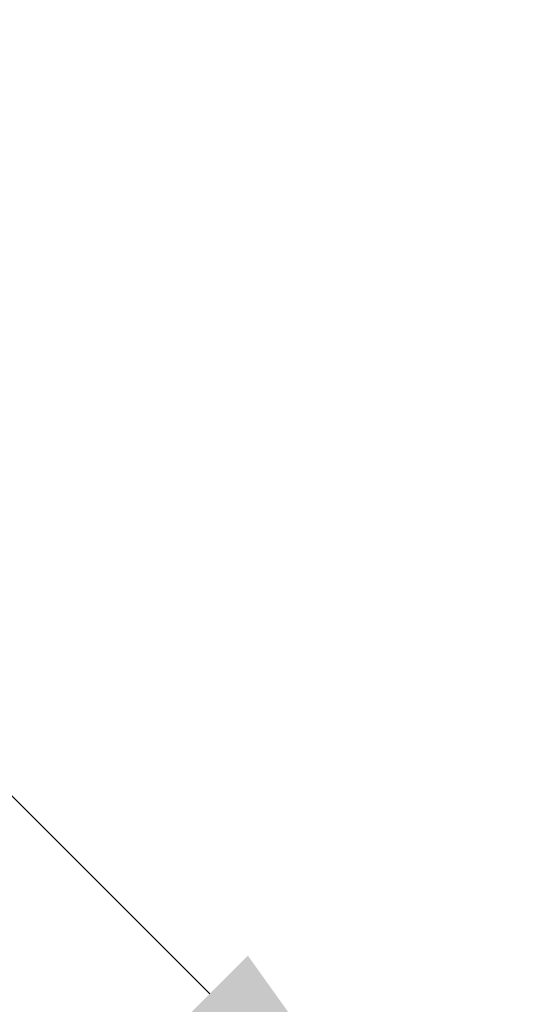
# Model space of a CAD drawing. Units: millimetres. Extents: x 0 to 2267, y 0 to 1823.
# Tile 16 of 256: x 1518.68 to 1525.06, y 1127.19 to 1139.34. Entities that reach past the tile are written whole.
import ezdxf

# ---------------------------------------------------------------- set-up
doc = ezdxf.new("R2010")
doc.units = ezdxf.units.MM
doc.header["$MEASUREMENT"] = 0
for name, color, linetype, lineweight in [('M-DIMS', 2, 'Continuous', 25), ('M-HATC', 252, 'Continuous', 18), ('M-OUTL', 7, 'Continuous', 50)]:
    doc.layers.add(name, color=color, linetype=linetype, lineweight=lineweight)
doc.styles.get("Standard").update_dxf_attribs({"font": 'arial.ttf'})
doc.dimstyles.get("Standard").update_dxf_attribs({"dimtxt": 7, "dimasz": 4, "dimexe": 0.18, "dimexo": 0.0625, "dimgap": 0.09, "dimtad": 0, "dimdec": 0, "dimzin": 0, "dimdsep": 46, "dimtxsty": 'Standard', "dimcen": 0.09, "dimadec": 0, "dimazin": 0, "dimtfac": 1, "dimtdec": 0, "dimtofl": 0, "dimtmove": 0, "dimatfit": 3, "dimfxl": 1, "dimtolj": 1, "dimtzin": 0, "dimarcsym": 0})

# ---------------------------------------------------------------- blocks, each defined once
blk = doc.blocks.new('*D28')
at = {"layer": 'Defpoints', "color": 0, "transparency": 16777216}
for p in [(1523.858, 1124.488), (1530.929, 1117.417)]:
    blk.add_point(p, dxfattribs=at)
at = {"layer": 'M-DIMS', "color": 0, "lineweight": -2, "transparency": 16777216}
for p, q in [((1518.201, 1130.145), (1521.029, 1127.317)), ((1530.929, 1117.327), (1530.929, 1117.507)), ((1530.839, 1117.417), (1531.019, 1117.417))]:
    blk.add_line(p, q, dxfattribs=at)
at = {"layer": 'M-DIMS', "color": 0, "transparency": 16777216}
blk.add_solid([(1521.501, 1127.788), (1520.558, 1126.845), (1523.858, 1124.488)], dxfattribs=at)
at = {"layer": 'M-DIMS', "color": 0, "transparency": 16777216, "insert": (1504.949, 1143.397), "char_height": 7, "attachment_point": 5, "rotation": 314.9998}
blk.add_mtext('\\A1;27X R10', dxfattribs=at)

msp = doc.modelspace()

# ---------------------------------------------------------------- hatches: boundary and pattern name
at = {"layer": 'M-HATC'}
h = msp.add_hatch(color=256, dxfattribs=at)
h.dxf.hatch_style = 1
h.paths.add_polyline_path([(2055.771, 1603.062), (1381.087, 1603.062), (1381.087, 1598.062), (2055.771, 1598.062)])
h.paths.add_polyline_path([(2055.771, 1598.062), (1381.087, 1598.062), (1381.087, 1593.062), (2055.771, 1593.062)])
h.paths.add_polyline_path([(2051.307, 1536.761), (1385.55, 1536.761), (1385.55, 1526.761), (1387.55, 1526.761), (1388.537, 1525.053), (1385.332, 1521.233), (1385.332, 1521.223), (2050.254, 1522.749), (2048.321, 1525.053), (2049.307, 1526.761), (2051.307, 1526.761)])
edge = h.paths.add_edge_path()
edge.add_arc((1847.535, 1379.149), 135, 222.60306, 222.89085, ccw=False)
edge.add_line((1748.166, 1287.766), (1683.092, 1287.766))
edge.add_arc((1583.724, 1379.149), 135, 317.10915, 317.39694, ccw=False)
edge.add_arc((1678.969, 1290.671), 5, 222.8909, 317.1091, ccw=False)
edge.add_arc((1774.213, 1379.149), 135, 222.60306, 222.89085, ccw=False)
edge.add_line((1674.845, 1287.766), (1609.771, 1287.766))
edge.add_arc((1510.403, 1379.149), 135, 317.10915, 317.39694, ccw=False)
edge.add_arc((1605.647, 1290.671), 5, 222.8909, 317.1091, ccw=False)
edge.add_arc((1700.892, 1379.149), 135, 222.60306, 222.89085, ccw=False)
edge.add_line((1601.524, 1287.766), (1536.45, 1287.766))
edge.add_arc((1437.081, 1379.149), 135, 317.10915, 317.39694, ccw=False)
edge.add_arc((1532.326, 1290.671), 5, 222.8909, 317.1091, ccw=False)
edge.add_arc((1627.571, 1379.149), 135, 222.60306, 222.89085, ccw=False)
edge.add_line((1528.203, 1287.766), (1505.929, 1287.766))
edge.add_spline(control_points=[(1505.929, 1287.766), (1504.262, 1287.766), (1504.262, 1282.766), (1505.929, 1282.766)], knot_values=[0, 0, 0, 0, 5, 5, 5, 5], degree=3, periodic=0)
edge.add_line((1505.929, 1282.766), (1930.929, 1282.766))
edge.add_spline(control_points=[(1930.929, 1282.766), (1932.596, 1282.766), (1932.596, 1287.766), (1930.929, 1287.766)], knot_values=[0, 0, 0, 0, 5, 5, 5, 5], degree=3, periodic=0)
edge.add_line((1930.929, 1287.766), (1903.056, 1287.766))
edge.add_arc((1803.688, 1379.149), 135, 317.10915, 317.39694, ccw=False)
edge.add_arc((1898.932, 1290.671), 5, 222.8909, 317.1091, ccw=False)
edge.add_arc((1994.177, 1379.149), 135, 222.60306, 222.89085, ccw=False)
edge.add_line((1894.809, 1287.766), (1829.735, 1287.766))
edge.add_arc((1730.366, 1379.149), 135, 317.10915, 317.39694, ccw=False)
edge.add_arc((1825.611, 1290.671), 5, 222.8909, 317.1091, ccw=False)
edge.add_arc((1920.856, 1379.149), 135, 222.60306, 222.89085, ccw=False)
edge.add_line((1821.487, 1287.766), (1756.413, 1287.766))
edge.add_arc((1657.045, 1379.149), 135, 317.10915, 317.39694, ccw=False)
edge.add_arc((1752.29, 1290.671), 5, 222.8909, 317.1091, ccw=False)
edge = h.paths.add_edge_path()
edge.add_spline(control_points=[(1843.429, 1227.247), (1845.096, 1227.247), (1845.096, 1232.247), (1843.429, 1232.247)], knot_values=[0, 0, 0, 0, 5, 5, 5, 5], degree=3, periodic=0)
edge.add_line((1843.429, 1232.247), (1593.429, 1232.247))
edge.add_spline(control_points=[(1593.429, 1232.247), (1591.762, 1232.247), (1591.762, 1227.247), (1593.429, 1227.247)], knot_values=[0, 0, 0, 0, 5, 5, 5, 5], degree=3, periodic=0)
edge.add_line((1593.429, 1227.247), (1843.429, 1227.247))
h.paths.add_polyline_path([(1905.929, 1127.417), (1530.929, 1127.417, 0.414214), (1520.929, 1117.417), (1530.929, 1117.417), (1915.929, 1117.417, 0.414214)])
edge = h.paths.add_edge_path()
edge.add_arc((1397.086, 1498.408), 12.73, 90.7821, 190.8787, ccw=False)
edge.add_line((1396.912, 1511.136), (1428.01, 1511.349))
edge.add_line((1428.01, 1511.349), (1433.01, 1511.349))
edge.add_line((1433.01, 1511.349), (1434.439, 1511.349))
edge.add_arc((1419.474, 1498.08), 20, 41.561, 74.0821)
edge.add_line((1424.959, 1517.314), (1399.935, 1517.256))
edge.add_spline(control_points=[(1399.931, 1517.256), (1399.884, 1517.213), (1399.833, 1517.169), (1399.777, 1517.124)], knot_values=[11.567499, 11.567499, 11.567499, 11.567499, 11.814249, 11.814249, 11.814249, 11.814249], degree=3, periodic=0)
edge.add_spline(control_points=[(1399.633, 1517.01), (1399.583, 1516.972), (1399.531, 1516.934), (1399.476, 1516.895)], knot_values=[11.167718, 11.167718, 11.167718, 11.167718, 11.365188, 11.365188, 11.365188, 11.365188], degree=3, periodic=0)
edge.add_spline(control_points=[(1399.34, 1516.8), (1399.151, 1516.672), (1398.938, 1516.538), (1398.704, 1516.399)], knot_values=[10.376405, 10.376405, 10.376405, 10.376405, 11.00994, 11.00994, 11.00994, 11.00994], degree=3, periodic=0)
edge.add_spline(control_points=[(1398.657, 1516.372), (1398.579, 1516.326), (1398.498, 1516.28), (1398.415, 1516.233)], knot_values=[10.125175, 10.125175, 10.125175, 10.125175, 10.334406, 10.334406, 10.334406, 10.334406], degree=3, periodic=0)
edge.add_spline(control_points=[(1398.264, 1516.149), (1398.196, 1516.111), (1398.126, 1516.073), (1398.055, 1516.035)], knot_values=[9.832246, 9.832246, 9.832246, 9.832246, 9.999658, 9.999658, 9.999658, 9.999658], degree=3, periodic=0)
edge.add_spline(control_points=[(1397.999, 1516.005), (1397.731, 1515.862), (1397.446, 1515.717), (1397.147, 1515.571)], knot_values=[9.161808, 9.161808, 9.161808, 9.161808, 9.787769, 9.787769, 9.787769, 9.787769], degree=3, periodic=0)
edge.add_spline(control_points=[(1397.147, 1515.571), (1396.842, 1515.423), (1396.522, 1515.274), (1396.191, 1515.126)], knot_values=[8.524455, 8.524455, 8.524455, 8.524455, 9.161808, 9.161808, 9.161808, 9.161808], degree=3, periodic=0)
edge.add_spline(control_points=[(1396.078, 1515.076), (1395.985, 1515.035), (1395.892, 1514.994), (1395.798, 1514.953)], knot_values=[8.275193, 8.275193, 8.275193, 8.275193, 8.451726, 8.451726, 8.451726, 8.451726], degree=3, periodic=0)
edge.add_spline(control_points=[(1395.602, 1514.869), (1395.5, 1514.826), (1395.397, 1514.782), (1395.293, 1514.739)], knot_values=[7.962917, 7.962917, 7.962917, 7.962917, 8.152764, 8.152764, 8.152764, 8.152764], degree=3, periodic=0)
edge.add_spline(control_points=[(1395.212, 1514.706), (1394.828, 1514.547), (1394.435, 1514.393), (1394.036, 1514.244)], knot_values=[7.21254, 7.21254, 7.21254, 7.21254, 7.913148, 7.913148, 7.913148, 7.913148], degree=3, periodic=0)
edge.add_spline(control_points=[(1394.036, 1514.244), (1393.708, 1514.121), (1393.375, 1514.003), (1393.043, 1513.889)], knot_values=[6.633733, 6.633733, 6.633733, 6.633733, 7.21254, 7.21254, 7.21254, 7.21254], degree=3, periodic=0)
edge.add_spline(control_points=[(1392.821, 1513.815), (1392.72, 1513.781), (1392.618, 1513.748), (1392.517, 1513.715)], knot_values=[6.328796, 6.328796, 6.328796, 6.328796, 6.505493, 6.505493, 6.505493, 6.505493], degree=3, periodic=0)
edge.add_spline(control_points=[(1392.517, 1513.715), (1392.319, 1513.652), (1392.121, 1513.59), (1391.924, 1513.531)], knot_values=[5.984605, 5.984605, 5.984605, 5.984605, 6.328796, 6.328796, 6.328796, 6.328796], degree=3, periodic=0)
edge.add_spline(control_points=[(1391.792, 1513.491), (1391.312, 1513.35), (1390.838, 1513.224), (1390.378, 1513.117)], knot_values=[5.066697, 5.066697, 5.066697, 5.066697, 5.907055, 5.907055, 5.907055, 5.907055], degree=3, periodic=0)
edge.add_spline(control_points=[(1390.378, 1513.117), (1390.18, 1513.071), (1389.984, 1513.028), (1389.791, 1512.99)], knot_values=[4.70367, 4.70367, 4.70367, 4.70367, 5.066695, 5.066695, 5.066695, 5.066695], degree=3, periodic=0)
edge.add_spline(control_points=[(1389.422, 1512.92), (1389.246, 1512.889), (1389.073, 1512.862), (1388.904, 1512.838)], knot_values=[4.130571, 4.130571, 4.130571, 4.130571, 4.469816, 4.469816, 4.469816, 4.469816], degree=3, periodic=0)
edge.add_spline(control_points=[(1388.904, 1512.838), (1388.591, 1512.795), (1388.291, 1512.764), (1388.007, 1512.749)], knot_values=[3.504031, 3.504031, 3.504031, 3.504031, 4.130571, 4.130571, 4.130571, 4.130571], degree=3, periodic=0)
edge.add_spline(control_points=[(1387.936, 1512.746), (1387.854, 1512.742), (1387.773, 1512.74), (1387.694, 1512.739)], knot_values=[3.268866, 3.268866, 3.268866, 3.268866, 3.451164, 3.451164, 3.451164, 3.451164], degree=3, periodic=0)
edge.add_spline(control_points=[(1387.335, 1512.744), (1387.208, 1512.75), (1387.085, 1512.76), (1386.967, 1512.774)], knot_values=[2.670686, 2.670686, 2.670686, 2.670686, 2.984, 2.984, 2.984, 2.984], degree=3, periodic=0)
edge.add_spline(control_points=[(1386.833, 1512.792), (1386.821, 1512.794), (1386.809, 1512.796), (1386.797, 1512.798)], knot_values=[2.516981, 2.516981, 2.516981, 2.516981, 2.549528, 2.549528, 2.549528, 2.549528], degree=3, periodic=0)
edge.add_spline(control_points=[(1386.453, 1512.873), (1386.426, 1512.881), (1386.399, 1512.889), (1386.373, 1512.897)], knot_values=[2.095869, 2.095869, 2.095869, 2.095869, 2.17941, 2.17941, 2.17941, 2.17941], degree=3, periodic=0)
edge.add_spline(control_points=[(1386.069, 1513.019), (1386.063, 1513.022), (1386.058, 1513.025), (1386.052, 1513.028)], knot_values=[1.72453, 1.72453, 1.72453, 1.72453, 1.745933, 1.745933, 1.745933, 1.745933], degree=3, periodic=0)
edge.add_arc((1399.474, 1498.08), 20, 131.8243, 180)
edge.add_arc((1630.334, 1505.548), 250.971, 181.70518, 236.42798)
edge.add_arc((1605.34, 1483.304), 218.782, 238.66083, 243.34961)
edge.add_arc((1647.091, 1510.359), 262.899, 183.12984, 237.85344, ccw=False)
h.paths.add_polyline_path([(1406.537, 1391.964, 0.149382), (1491.551, 1296.442, -0.129517)], flags=17)
edge = h.paths.add_edge_path()
edge.add_arc((2037.384, 1498.08), 20, 0, 48.2659)
edge.add_spline(control_points=[(2050.697, 1513.005), (2050.651, 1512.985), (2050.603, 1512.966), (2050.554, 1512.948)], knot_values=[1.835652, 1.835652, 1.835652, 1.835652, 2.000781, 2.000781, 2.000781, 2.000781], degree=3, periodic=0)
edge.add_spline(control_points=[(2050.462, 1512.917), (2050.479, 1512.922), (2050.496, 1512.928), (2050.513, 1512.934)], knot_values=[2.045477, 2.045477, 2.045477, 2.045477, 2.101389, 2.101389, 2.101389, 2.101389], degree=3, periodic=0)
edge.add_spline(control_points=[(2050.129, 1512.834), (2050.198, 1512.847), (2050.266, 1512.862), (2050.331, 1512.879)], knot_values=[2.237629, 2.237629, 2.237629, 2.237629, 2.435841, 2.435841, 2.435841, 2.435841], degree=3, periodic=0)
edge.add_spline(control_points=[(2050.095, 1512.828), (2050.106, 1512.83), (2050.118, 1512.832), (2050.129, 1512.834)], knot_values=[2.435841, 2.435841, 2.435841, 2.435841, 2.468321, 2.468321, 2.468321, 2.468321], degree=3, periodic=0)
edge.add_spline(control_points=[(2049.784, 1512.785), (2049.855, 1512.792), (2049.924, 1512.801), (2049.992, 1512.811)], knot_values=[2.563852, 2.563852, 2.563852, 2.563852, 2.748541, 2.748541, 2.748541, 2.748541], degree=3, periodic=0)
edge.add_spline(control_points=[(2049.405, 1512.762), (2049.536, 1512.765), (2049.663, 1512.773), (2049.784, 1512.785)], knot_values=[2.748541, 2.748541, 2.748541, 2.748541, 3.064882, 3.064882, 3.064882, 3.064882], degree=3, periodic=0)
edge.add_spline(control_points=[(2049.17, 1512.76), (2049.234, 1512.759), (2049.297, 1512.759), (2049.358, 1512.761)], knot_values=[3.102309, 3.102309, 3.102309, 3.102309, 3.2503, 3.2503, 3.2503, 3.2503], degree=3, periodic=0)
edge.add_spline(control_points=[(2048.857, 1512.769), (2048.964, 1512.764), (2049.068, 1512.761), (2049.17, 1512.76)], knot_values=[3.2503, 3.2503, 3.2503, 3.2503, 3.486069, 3.486069, 3.486069, 3.486069], degree=3, periodic=0)
edge.add_spline(control_points=[(2048.692, 1512.779), (2048.373, 1512.801), (2048.035, 1512.841), (2047.682, 1512.897)], knot_values=[3.606429, 3.606429, 3.606429, 3.606429, 4.2989, 4.2989, 4.2989, 4.2989], degree=3, periodic=0)
edge.add_spline(control_points=[(2047.682, 1512.897), (2047.546, 1512.919), (2047.408, 1512.942), (2047.268, 1512.969)], knot_values=[4.2989, 4.2989, 4.2989, 4.2989, 4.565769, 4.565769, 4.565769, 4.565769], degree=3, periodic=0)
edge.add_spline(control_points=[(2047.268, 1512.969), (2047.145, 1512.991), (2047.021, 1513.016), (2046.895, 1513.042)], knot_values=[4.565769, 4.565769, 4.565769, 4.565769, 4.799971, 4.799971, 4.799971, 4.799971], degree=3, periodic=0)
edge.add_spline(control_points=[(2046.895, 1513.042), (2046.529, 1513.119), (2046.151, 1513.209), (2045.768, 1513.311)], knot_values=[4.799971, 4.799971, 4.799971, 4.799971, 5.483718, 5.483718, 5.483718, 5.483718], degree=3, periodic=0)
edge.add_spline(control_points=[(2045.768, 1513.311), (2045.372, 1513.415), (2044.97, 1513.532), (2044.566, 1513.659)], knot_values=[5.483718, 5.483718, 5.483718, 5.483718, 6.187866, 6.187866, 6.187866, 6.187866], degree=3, periodic=0)
edge.add_spline(control_points=[(2044.566, 1513.659), (2044.415, 1513.706), (2044.263, 1513.755), (2044.112, 1513.805)], knot_values=[6.187866, 6.187866, 6.187866, 6.187866, 6.451551, 6.451551, 6.451551, 6.451551], degree=3, periodic=0)
edge.add_spline(control_points=[(2044.112, 1513.805), (2043.997, 1513.843), (2043.882, 1513.881), (2043.767, 1513.92)], knot_values=[6.451551, 6.451551, 6.451551, 6.451551, 6.651434, 6.651434, 6.651434, 6.651434], degree=3, periodic=0)
edge.add_spline(control_points=[(2043.767, 1513.92), (2043.372, 1514.055), (2042.977, 1514.198), (2042.589, 1514.346)], knot_values=[6.651434, 6.651434, 6.651434, 6.651434, 7.338879, 7.338879, 7.338879, 7.338879], degree=3, periodic=0)
edge.add_spline(control_points=[(2042.589, 1514.346), (2042.164, 1514.507), (2041.746, 1514.675), (2041.341, 1514.846)], knot_values=[7.338879, 7.338879, 7.338879, 7.338879, 8.089209, 8.089209, 8.089209, 8.089209], degree=3, periodic=0)
edge.add_spline(control_points=[(2041.341, 1514.846), (2041.103, 1514.946), (2040.869, 1515.048), (2040.64, 1515.15)], knot_values=[8.089209, 8.089209, 8.089209, 8.089209, 8.529587, 8.529587, 8.529587, 8.529587], degree=3, periodic=0)
edge.add_spline(control_points=[(2040.51, 1515.209), (2040.082, 1515.402), (2039.675, 1515.597), (2039.295, 1515.789)], knot_values=[8.613818, 8.613818, 8.613818, 8.613818, 9.44571, 9.44571, 9.44571, 9.44571], degree=3, periodic=0)
edge.add_spline(control_points=[(2039.295, 1515.789), (2039.062, 1515.907), (2038.839, 1516.025), (2038.629, 1516.14)], knot_values=[9.44571, 9.44571, 9.44571, 9.44571, 9.956404, 9.956404, 9.956404, 9.956404], degree=3, periodic=0)
edge.add_spline(control_points=[(2038.629, 1516.14), (2038.519, 1516.2), (2038.412, 1516.26), (2038.309, 1516.319)], knot_values=[9.956404, 9.956404, 9.956404, 9.956404, 10.223542, 10.223542, 10.223542, 10.223542], degree=3, periodic=0)
edge.add_spline(control_points=[(2038.309, 1516.319), (2038.214, 1516.374), (2038.122, 1516.428), (2038.033, 1516.481)], knot_values=[10.223542, 10.223542, 10.223542, 10.223542, 10.47051, 10.47051, 10.47051, 10.47051], degree=3, periodic=0)
edge.add_spline(control_points=[(2038.033, 1516.481), (2037.786, 1516.63), (2037.564, 1516.773), (2037.372, 1516.909)], knot_values=[10.47051, 10.47051, 10.47051, 10.47051, 11.15767, 11.15767, 11.15767, 11.15767], degree=3, periodic=0)
edge.add_spline(control_points=[(2037.372, 1516.909), (2037.279, 1516.975), (2037.193, 1517.04), (2037.114, 1517.102)], knot_values=[11.15767, 11.15767, 11.15767, 11.15767, 11.49227, 11.49227, 11.49227, 11.49227], degree=3, periodic=0)
edge.add_spline(control_points=[(2036.856, 1517.326), (2036.915, 1517.269), (2036.981, 1517.21), (2037.056, 1517.149)], knot_values=[11.577341, 11.577341, 11.577341, 11.577341, 11.91035, 11.91035, 11.91035, 11.91035], degree=3, periodic=0)
edge.add_spline(control_points=[(2036.807, 1517.375), (2036.823, 1517.359), (2036.839, 1517.342), (2036.856, 1517.326)], knot_values=[11.91035, 11.91035, 11.91035, 11.91035, 12.007402, 12.007402, 12.007402, 12.007402], degree=3, periodic=0)
edge.add_spline(control_points=[(2036.702, 1517.494), (2036.71, 1517.483), (2036.72, 1517.472), (2036.729, 1517.461)], knot_values=[12.184155, 12.184155, 12.184155, 12.184155, 12.255409, 12.255409, 12.255409, 12.255409], degree=3, periodic=0)
edge.add_spline(control_points=[(2036.616, 1517.621), (2036.62, 1517.613), (2036.624, 1517.606), (2036.629, 1517.598)], knot_values=[12.487913, 12.487913, 12.487913, 12.487913, 12.541035, 12.541035, 12.541035, 12.541035], degree=3, periodic=0)
edge.add_spline(control_points=[(2036.563, 1517.786), (2036.564, 1517.779), (2036.564, 1517.773), (2036.565, 1517.766)], knot_values=[12.911761, 12.911761, 12.911761, 12.911761, 12.968286, 12.968286, 12.968286, 12.968286], degree=3, periodic=0)
edge.add_spline(control_points=[(2036.617, 1517.93), (2036.612, 1517.926), (2036.609, 1517.921), (2036.605, 1517.916)], knot_values=[13.382527, 13.382527, 13.382527, 13.382527, 13.433791, 13.433791, 13.433791, 13.433791], degree=3, periodic=0)
edge.add_spline(control_points=[(2036.749, 1518.017), (2036.736, 1518.012), (2036.724, 1518.006), (2036.712, 1518)], knot_values=[13.726299, 13.726299, 13.726299, 13.726299, 13.809928, 13.809928, 13.809928, 13.809928], degree=3, periodic=0)
edge.add_spline(control_points=[(2036.86, 1518.053), (2036.839, 1518.047), (2036.818, 1518.042), (2036.799, 1518.035)], knot_values=[13.910887, 13.910887, 13.910887, 13.910887, 14.02153, 14.02153, 14.02153, 14.02153], degree=3, periodic=0)
edge.add_line((2036.964, 1518.08), (2032.384, 1518.08))
edge.add_line((2032.384, 1518.08), (2027.384, 1518.08))
edge.add_line((2027.384, 1518.08), (2022.384, 1518.08))
edge.add_line((2022.384, 1518.08), (2017.384, 1518.08))
edge.add_arc((2017.384, 1498.08), 20, 90, 138.439)
edge.add_line((2002.419, 1511.349), (2003.848, 1511.349))
edge.add_line((2003.848, 1511.349), (2008.848, 1511.349))
edge.add_line((2008.848, 1511.349), (2039.772, 1511.138))
edge.add_arc((2039.772, 1498.408), 12.73, -10.8787, 90, ccw=False)
edge.add_arc((1789.767, 1510.359), 262.899, 302.14656, 356.87016, ccw=False)
edge.add_arc((1831.518, 1483.304), 218.782, 296.65039, 301.33917)
edge.add_arc((1806.524, 1505.548), 250.971, 303.57202, 358.29482)
h.paths.add_polyline_path([(2030.321, 1391.964, -0.129517), (1945.307, 1296.442, 0.149382)], flags=17)
edge = h.paths.add_edge_path()
edge.add_spline(control_points=[(2037.246, 1518.082), (2037.29, 1518.081), (2037.336, 1518.08), (2037.384, 1518.08)], knot_values=[0.000012, 0.000012, 0.000012, 0.000012, 0.144754, 0.144754, 0.144754, 0.144754], degree=3, periodic=0)
edge.add_line((2037.336, 1518.08), (2037.01, 1518.08))
edge.add_spline(control_points=[(2037.01, 1518.08), (2036.982, 1518.077), (2036.956, 1518.073), (2036.931, 1518.068)], knot_values=[14.13465, 14.13465, 14.13465, 14.13465, 14.247197, 14.247197, 14.247197, 14.247197], degree=3, periodic=0)
edge.add_spline(control_points=[(2036.931, 1518.068), (2036.928, 1518.067), (2036.924, 1518.067), (2036.921, 1518.066)], knot_values=[14.118315, 14.118315, 14.118315, 14.118315, 14.13465, 14.13465, 14.13465, 14.13465], degree=3, periodic=0)
edge.add_spline(control_points=[(2036.921, 1518.066), (2036.912, 1518.064), (2036.903, 1518.063), (2036.895, 1518.061)], knot_values=[14.078086, 14.078086, 14.078086, 14.078086, 14.118315, 14.118315, 14.118315, 14.118315], degree=3, periodic=0)
edge.add_spline(control_points=[(2036.895, 1518.061), (2036.883, 1518.058), (2036.872, 1518.056), (2036.86, 1518.053)], knot_values=[14.02153, 14.02153, 14.02153, 14.02153, 14.078086, 14.078086, 14.078086, 14.078086], degree=3, periodic=0)
edge.add_spline(control_points=[(2036.86, 1518.053), (2036.839, 1518.047), (2036.818, 1518.042), (2036.799, 1518.035)], knot_values=[13.910887, 13.910887, 13.910887, 13.910887, 14.02153, 14.02153, 14.02153, 14.02153], degree=3, periodic=0)
edge.add_spline(control_points=[(2036.799, 1518.035), (2036.798, 1518.035), (2036.797, 1518.035), (2036.797, 1518.035)], knot_values=[13.906906, 13.906906, 13.906906, 13.906906, 13.910887, 13.910887, 13.910887, 13.910887], degree=3, periodic=0)
edge.add_spline(control_points=[(2036.797, 1518.035), (2036.788, 1518.032), (2036.78, 1518.029), (2036.772, 1518.026)], knot_values=[13.857826, 13.857826, 13.857826, 13.857826, 13.906906, 13.906906, 13.906906, 13.906906], degree=3, periodic=0)
edge.add_spline(control_points=[(2036.772, 1518.026), (2036.764, 1518.023), (2036.756, 1518.02), (2036.749, 1518.017)], knot_values=[13.809928, 13.809928, 13.809928, 13.809928, 13.857826, 13.857826, 13.857826, 13.857826], degree=3, periodic=0)
edge.add_spline(control_points=[(2036.749, 1518.017), (2036.736, 1518.012), (2036.724, 1518.006), (2036.712, 1518)], knot_values=[13.726299, 13.726299, 13.726299, 13.726299, 13.809928, 13.809928, 13.809928, 13.809928], degree=3, periodic=0)
edge.add_spline(control_points=[(2036.712, 1518), (2036.712, 1518), (2036.712, 1518), (2036.711, 1518)], knot_values=[13.723993, 13.723993, 13.723993, 13.723993, 13.726299, 13.726299, 13.726299, 13.726299], degree=3, periodic=0)
edge.add_spline(control_points=[(2036.711, 1518), (2036.706, 1517.997), (2036.701, 1517.994), (2036.696, 1517.992)], knot_values=[13.686536, 13.686536, 13.686536, 13.686536, 13.723993, 13.723993, 13.723993, 13.723993], degree=3, periodic=0)
edge.add_spline(control_points=[(2036.696, 1517.992), (2036.692, 1517.989), (2036.687, 1517.987), (2036.683, 1517.984)], knot_values=[13.651251, 13.651251, 13.651251, 13.651251, 13.686536, 13.686536, 13.686536, 13.686536], degree=3, periodic=0)
edge.add_spline(control_points=[(2036.683, 1517.984), (2036.676, 1517.98), (2036.67, 1517.976), (2036.664, 1517.971)], knot_values=[13.596804, 13.596804, 13.596804, 13.596804, 13.651251, 13.651251, 13.651251, 13.651251], degree=3, periodic=0)
edge.add_spline(control_points=[(2036.664, 1517.971), (2036.664, 1517.971), (2036.663, 1517.971), (2036.663, 1517.971)], knot_values=[13.593956, 13.593956, 13.593956, 13.593956, 13.596804, 13.596804, 13.596804, 13.596804], degree=3, periodic=0)
edge.add_spline(control_points=[(2036.663, 1517.971), (2036.66, 1517.969), (2036.658, 1517.967), (2036.655, 1517.965)], knot_values=[13.570322, 13.570322, 13.570322, 13.570322, 13.593956, 13.593956, 13.593956, 13.593956], degree=3, periodic=0)
edge.add_spline(control_points=[(2036.655, 1517.965), (2036.653, 1517.963), (2036.65, 1517.961), (2036.647, 1517.959)], knot_values=[13.545477, 13.545477, 13.545477, 13.545477, 13.570322, 13.570322, 13.570322, 13.570322], degree=3, periodic=0)
edge.add_spline(control_points=[(2036.647, 1517.959), (2036.647, 1517.959), (2036.647, 1517.959), (2036.647, 1517.959)], knot_values=[13.543931, 13.543931, 13.543931, 13.543931, 13.545477, 13.545477, 13.545477, 13.545477], degree=3, periodic=0)
edge.add_spline(control_points=[(2036.647, 1517.959), (2036.641, 1517.954), (2036.636, 1517.949), (2036.631, 1517.945)], knot_values=[13.488237, 13.488237, 13.488237, 13.488237, 13.543931, 13.543931, 13.543931, 13.543931], degree=3, periodic=0)
edge.add_spline(control_points=[(2036.631, 1517.945), (2036.628, 1517.942), (2036.626, 1517.94), (2036.623, 1517.937)], knot_values=[13.460307, 13.460307, 13.460307, 13.460307, 13.488237, 13.488237, 13.488237, 13.488237], degree=3, periodic=0)
edge.add_spline(control_points=[(2036.623, 1517.937), (2036.622, 1517.936), (2036.62, 1517.934), (2036.618, 1517.932)], knot_values=[13.439712, 13.439712, 13.439712, 13.439712, 13.460307, 13.460307, 13.460307, 13.460307], degree=3, periodic=0)
edge.add_spline(control_points=[(2036.618, 1517.932), (2036.618, 1517.931), (2036.617, 1517.931), (2036.617, 1517.93)], knot_values=[13.433791, 13.433791, 13.433791, 13.433791, 13.439712, 13.439712, 13.439712, 13.439712], degree=3, periodic=0)
edge.add_spline(control_points=[(2036.617, 1517.93), (2036.612, 1517.926), (2036.609, 1517.921), (2036.605, 1517.916)], knot_values=[13.382527, 13.382527, 13.382527, 13.382527, 13.433791, 13.433791, 13.433791, 13.433791], degree=3, periodic=0)
edge.add_spline(control_points=[(2036.605, 1517.916), (2036.603, 1517.913), (2036.6, 1517.91), (2036.598, 1517.907)], knot_values=[13.350017, 13.350017, 13.350017, 13.350017, 13.382527, 13.382527, 13.382527, 13.382527], degree=3, periodic=0)
edge.add_spline(control_points=[(2036.598, 1517.907), (2036.597, 1517.906), (2036.596, 1517.904), (2036.595, 1517.903)], knot_values=[13.333922, 13.333922, 13.333922, 13.333922, 13.350017, 13.350017, 13.350017, 13.350017], degree=3, periodic=0)
edge.add_spline(control_points=[(2036.595, 1517.903), (2036.595, 1517.902), (2036.594, 1517.901), (2036.593, 1517.9)], knot_values=[13.323828, 13.323828, 13.323828, 13.323828, 13.333922, 13.333922, 13.333922, 13.333922], degree=3, periodic=0)
edge.add_spline(control_points=[(2036.593, 1517.9), (2036.59, 1517.895), (2036.588, 1517.891), (2036.585, 1517.886)], knot_values=[13.277545, 13.277545, 13.277545, 13.277545, 13.323828, 13.323828, 13.323828, 13.323828], degree=3, periodic=0)
edge.add_spline(control_points=[(2036.585, 1517.886), (2036.584, 1517.883), (2036.582, 1517.879), (2036.58, 1517.875)], knot_values=[13.240119, 13.240119, 13.240119, 13.240119, 13.277545, 13.277545, 13.277545, 13.277545], degree=3, periodic=0)
edge.add_spline(control_points=[(2036.58, 1517.875), (2036.58, 1517.874), (2036.579, 1517.873), (2036.578, 1517.872)], knot_values=[13.228211, 13.228211, 13.228211, 13.228211, 13.240119, 13.240119, 13.240119, 13.240119], degree=3, periodic=0)
edge.add_spline(control_points=[(2036.578, 1517.872), (2036.578, 1517.87), (2036.577, 1517.869), (2036.577, 1517.868)], knot_values=[13.215717, 13.215717, 13.215717, 13.215717, 13.228211, 13.228211, 13.228211, 13.228211], degree=3, periodic=0)
edge.add_spline(control_points=[(2036.577, 1517.868), (2036.575, 1517.864), (2036.574, 1517.86), (2036.573, 1517.857)], knot_values=[13.179847, 13.179847, 13.179847, 13.179847, 13.215717, 13.215717, 13.215717, 13.215717], degree=3, periodic=0)
edge.add_spline(control_points=[(2036.573, 1517.857), (2036.571, 1517.851), (2036.57, 1517.846), (2036.569, 1517.841)], knot_values=[13.132017, 13.132017, 13.132017, 13.132017, 13.179847, 13.179847, 13.179847, 13.179847], degree=3, periodic=0)
edge.add_spline(control_points=[(2036.569, 1517.841), (2036.568, 1517.84), (2036.568, 1517.839), (2036.568, 1517.838)], knot_values=[13.122482, 13.122482, 13.122482, 13.122482, 13.132017, 13.132017, 13.132017, 13.132017], degree=3, periodic=0)
edge.add_spline(control_points=[(2036.568, 1517.838), (2036.568, 1517.836), (2036.567, 1517.835), (2036.567, 1517.833)], knot_values=[13.105592, 13.105592, 13.105592, 13.105592, 13.122482, 13.122482, 13.122482, 13.122482], degree=3, periodic=0)
edge.add_spline(control_points=[(2036.567, 1517.833), (2036.566, 1517.829), (2036.566, 1517.826), (2036.565, 1517.822)], knot_values=[13.074063, 13.074063, 13.074063, 13.074063, 13.105592, 13.105592, 13.105592, 13.105592], degree=3, periodic=0)
edge.add_spline(control_points=[(2036.565, 1517.822), (2036.565, 1517.822), (2036.565, 1517.822), (2036.565, 1517.822)], knot_values=[13.074043, 13.074043, 13.074043, 13.074043, 13.074063, 13.074063, 13.074063, 13.074063], degree=3, periodic=0)
edge.add_spline(control_points=[(2036.565, 1517.822), (2036.564, 1517.816), (2036.564, 1517.811), (2036.564, 1517.805)], knot_values=[13.021884, 13.021884, 13.021884, 13.021884, 13.074043, 13.074043, 13.074043, 13.074043], degree=3, periodic=0)
edge.add_spline(control_points=[(2036.564, 1517.805), (2036.564, 1517.804), (2036.564, 1517.803), (2036.564, 1517.803)], knot_values=[13.01674, 13.01674, 13.01674, 13.01674, 13.021884, 13.021884, 13.021884, 13.021884], degree=3, periodic=0)
edge.add_spline(control_points=[(2036.564, 1517.803), (2036.563, 1517.801), (2036.563, 1517.798), (2036.563, 1517.796)], knot_values=[12.996438, 12.996438, 12.996438, 12.996438, 13.01674, 13.01674, 13.01674, 13.01674], degree=3, periodic=0)
edge.add_spline(control_points=[(2036.563, 1517.796), (2036.563, 1517.793), (2036.563, 1517.789), (2036.563, 1517.786)], knot_values=[12.968286, 12.968286, 12.968286, 12.968286, 12.996438, 12.996438, 12.996438, 12.996438], degree=3, periodic=0)
edge.add_spline(control_points=[(2036.563, 1517.786), (2036.564, 1517.779), (2036.564, 1517.773), (2036.565, 1517.766)], knot_values=[12.911761, 12.911761, 12.911761, 12.911761, 12.968286, 12.968286, 12.968286, 12.968286], degree=3, periodic=0)
edge.add_spline(control_points=[(2036.565, 1517.766), (2036.565, 1517.766), (2036.565, 1517.766), (2036.565, 1517.766)], knot_values=[12.911017, 12.911017, 12.911017, 12.911017, 12.911761, 12.911761, 12.911761, 12.911761], degree=3, periodic=0)
edge.add_spline(control_points=[(2036.565, 1517.766), (2036.565, 1517.762), (2036.566, 1517.759), (2036.566, 1517.756)], knot_values=[12.88528, 12.88528, 12.88528, 12.88528, 12.911017, 12.911017, 12.911017, 12.911017], degree=3, periodic=0)
edge.add_spline(control_points=[(2036.566, 1517.756), (2036.567, 1517.753), (2036.567, 1517.751), (2036.568, 1517.748)], knot_values=[12.862519, 12.862519, 12.862519, 12.862519, 12.88528, 12.88528, 12.88528, 12.88528], degree=3, periodic=0)
edge.add_spline(control_points=[(2036.568, 1517.748), (2036.568, 1517.747), (2036.568, 1517.747), (2036.568, 1517.746)], knot_values=[12.858885, 12.858885, 12.858885, 12.858885, 12.862519, 12.862519, 12.862519, 12.862519], degree=3, periodic=0)
edge.add_spline(control_points=[(2036.568, 1517.746), (2036.569, 1517.74), (2036.571, 1517.733), (2036.572, 1517.726)], knot_values=[12.8053, 12.8053, 12.8053, 12.8053, 12.858885, 12.858885, 12.858885, 12.858885], degree=3, periodic=0)
edge.add_spline(control_points=[(2036.572, 1517.726), (2036.573, 1517.723), (2036.574, 1517.719), (2036.576, 1517.715)], knot_values=[12.775176, 12.775176, 12.775176, 12.775176, 12.8053, 12.8053, 12.8053, 12.8053], degree=3, periodic=0)
edge.add_spline(control_points=[(2036.576, 1517.715), (2036.576, 1517.713), (2036.577, 1517.71), (2036.578, 1517.708)], knot_values=[12.756759, 12.756759, 12.756759, 12.756759, 12.775176, 12.775176, 12.775176, 12.775176], degree=3, periodic=0)
edge.add_spline(control_points=[(2036.578, 1517.708), (2036.578, 1517.707), (2036.578, 1517.706), (2036.579, 1517.705)], knot_values=[12.748742, 12.748742, 12.748742, 12.748742, 12.756759, 12.756759, 12.756759, 12.756759], degree=3, periodic=0)
edge.add_spline(control_points=[(2036.579, 1517.705), (2036.581, 1517.698), (2036.583, 1517.692), (2036.586, 1517.685)], knot_values=[12.69959, 12.69959, 12.69959, 12.69959, 12.748742, 12.748742, 12.748742, 12.748742], degree=3, periodic=0)
edge.add_spline(control_points=[(2036.586, 1517.685), (2036.588, 1517.68), (2036.59, 1517.675), (2036.592, 1517.669)], knot_values=[12.659038, 12.659038, 12.659038, 12.659038, 12.69959, 12.69959, 12.69959, 12.69959], degree=3, periodic=0)
edge.add_spline(control_points=[(2036.592, 1517.669), (2036.594, 1517.665), (2036.596, 1517.66), (2036.598, 1517.656)], knot_values=[12.626806, 12.626806, 12.626806, 12.626806, 12.659038, 12.659038, 12.659038, 12.659038], degree=3, periodic=0)
edge.add_spline(control_points=[(2036.598, 1517.656), (2036.598, 1517.655), (2036.599, 1517.654), (2036.599, 1517.653)], knot_values=[12.619394, 12.619394, 12.619394, 12.619394, 12.626806, 12.626806, 12.626806, 12.626806], degree=3, periodic=0)
edge.add_spline(control_points=[(2036.599, 1517.653), (2036.604, 1517.642), (2036.61, 1517.632), (2036.616, 1517.621)], knot_values=[12.541039, 12.541039, 12.541039, 12.541039, 12.619394, 12.619394, 12.619394, 12.619394], degree=3, periodic=0)
edge.add_spline(control_points=[(2036.616, 1517.621), (2036.616, 1517.621), (2036.616, 1517.621), (2036.616, 1517.621)], knot_values=[12.541035, 12.541035, 12.541035, 12.541035, 12.541039, 12.541039, 12.541039, 12.541039], degree=3, periodic=0)
edge.add_spline(control_points=[(2036.616, 1517.621), (2036.62, 1517.613), (2036.624, 1517.606), (2036.629, 1517.598)], knot_values=[12.487913, 12.487913, 12.487913, 12.487913, 12.541035, 12.541035, 12.541035, 12.541035], degree=3, periodic=0)
edge.add_spline(control_points=[(2036.629, 1517.598), (2036.633, 1517.592), (2036.637, 1517.585), (2036.641, 1517.579)], knot_values=[12.443982, 12.443982, 12.443982, 12.443982, 12.487913, 12.487913, 12.487913, 12.487913], degree=3, periodic=0)
edge.add_spline(control_points=[(2036.641, 1517.579), (2036.641, 1517.578), (2036.642, 1517.576), (2036.643, 1517.575)], knot_values=[12.434996, 12.434996, 12.434996, 12.434996, 12.443982, 12.443982, 12.443982, 12.443982], degree=3, periodic=0)
edge.add_spline(control_points=[(2036.643, 1517.575), (2036.653, 1517.56), (2036.664, 1517.544), (2036.676, 1517.528)], knot_values=[12.329647, 12.329647, 12.329647, 12.329647, 12.434996, 12.434996, 12.434996, 12.434996], degree=3, periodic=0)
edge.add_spline(control_points=[(2036.676, 1517.528), (2036.684, 1517.517), (2036.693, 1517.505), (2036.702, 1517.494)], knot_values=[12.255409, 12.255409, 12.255409, 12.255409, 12.329647, 12.329647, 12.329647, 12.329647], degree=3, periodic=0)
edge.add_spline(control_points=[(2036.702, 1517.494), (2036.71, 1517.483), (2036.72, 1517.472), (2036.729, 1517.461)], knot_values=[12.184155, 12.184155, 12.184155, 12.184155, 12.255409, 12.255409, 12.255409, 12.255409], degree=3, periodic=0)
edge.add_spline(control_points=[(2036.729, 1517.461), (2036.744, 1517.444), (2036.759, 1517.426), (2036.775, 1517.409)], knot_values=[12.075961, 12.075961, 12.075961, 12.075961, 12.184155, 12.184155, 12.184155, 12.184155], degree=3, periodic=0)
edge.add_spline(control_points=[(2036.775, 1517.409), (2036.776, 1517.407), (2036.777, 1517.406), (2036.778, 1517.405)], knot_values=[12.069502, 12.069502, 12.069502, 12.069502, 12.075961, 12.075961, 12.075961, 12.075961], degree=3, periodic=0)
edge.add_spline(control_points=[(2036.778, 1517.405), (2036.788, 1517.395), (2036.797, 1517.385), (2036.807, 1517.375)], knot_values=[12.007402, 12.007402, 12.007402, 12.007402, 12.069502, 12.069502, 12.069502, 12.069502], degree=3, periodic=0)
edge.add_spline(control_points=[(2036.807, 1517.375), (2036.823, 1517.359), (2036.839, 1517.342), (2036.856, 1517.326)], knot_values=[11.91035, 11.91035, 11.91035, 11.91035, 12.007402, 12.007402, 12.007402, 12.007402], degree=3, periodic=0)
edge.add_spline(control_points=[(2036.856, 1517.326), (2036.915, 1517.269), (2036.981, 1517.21), (2037.056, 1517.149)], knot_values=[11.577341, 11.577341, 11.577341, 11.577341, 11.91035, 11.91035, 11.91035, 11.91035], degree=3, periodic=0)
edge.add_spline(control_points=[(2037.056, 1517.149), (2037.075, 1517.134), (2037.094, 1517.118), (2037.114, 1517.102)], knot_values=[11.49227, 11.49227, 11.49227, 11.49227, 11.577341, 11.577341, 11.577341, 11.577341], degree=3, periodic=0)
edge.add_spline(control_points=[(2037.114, 1517.102), (2037.193, 1517.04), (2037.279, 1516.975), (2037.372, 1516.909)], knot_values=[11.15767, 11.15767, 11.15767, 11.15767, 11.49227, 11.49227, 11.49227, 11.49227], degree=3, periodic=0)
edge.add_spline(control_points=[(2037.372, 1516.909), (2037.564, 1516.773), (2037.786, 1516.63), (2038.033, 1516.481)], knot_values=[10.47051, 10.47051, 10.47051, 10.47051, 11.15767, 11.15767, 11.15767, 11.15767], degree=3, periodic=0)
edge.add_spline(control_points=[(2038.033, 1516.481), (2038.122, 1516.428), (2038.214, 1516.374), (2038.309, 1516.319)], knot_values=[10.223542, 10.223542, 10.223542, 10.223542, 10.47051, 10.47051, 10.47051, 10.47051], degree=3, periodic=0)
edge.add_spline(control_points=[(2038.309, 1516.319), (2038.412, 1516.26), (2038.519, 1516.2), (2038.629, 1516.14)], knot_values=[9.956404, 9.956404, 9.956404, 9.956404, 10.223542, 10.223542, 10.223542, 10.223542], degree=3, periodic=0)
edge.add_spline(control_points=[(2038.629, 1516.14), (2038.839, 1516.025), (2039.062, 1515.907), (2039.295, 1515.789)], knot_values=[9.44571, 9.44571, 9.44571, 9.44571, 9.956404, 9.956404, 9.956404, 9.956404], degree=3, periodic=0)
edge.add_spline(control_points=[(2039.295, 1515.789), (2039.675, 1515.597), (2040.082, 1515.402), (2040.51, 1515.209)], knot_values=[8.613818, 8.613818, 8.613818, 8.613818, 9.44571, 9.44571, 9.44571, 9.44571], degree=3, periodic=0)
edge.add_spline(control_points=[(2040.51, 1515.209), (2040.553, 1515.189), (2040.597, 1515.17), (2040.64, 1515.15)], knot_values=[8.529587, 8.529587, 8.529587, 8.529587, 8.613818, 8.613818, 8.613818, 8.613818], degree=3, periodic=0)
edge.add_spline(control_points=[(2040.64, 1515.15), (2040.869, 1515.048), (2041.103, 1514.946), (2041.341, 1514.846)], knot_values=[8.089209, 8.089209, 8.089209, 8.089209, 8.529587, 8.529587, 8.529587, 8.529587], degree=3, periodic=0)
edge.add_spline(control_points=[(2041.341, 1514.846), (2041.746, 1514.675), (2042.164, 1514.507), (2042.589, 1514.346)], knot_values=[7.338879, 7.338879, 7.338879, 7.338879, 8.089209, 8.089209, 8.089209, 8.089209], degree=3, periodic=0)
edge.add_spline(control_points=[(2042.589, 1514.346), (2042.977, 1514.198), (2043.372, 1514.055), (2043.767, 1513.92)], knot_values=[6.651434, 6.651434, 6.651434, 6.651434, 7.338879, 7.338879, 7.338879, 7.338879], degree=3, periodic=0)
edge.add_spline(control_points=[(2043.767, 1513.92), (2043.882, 1513.881), (2043.997, 1513.843), (2044.112, 1513.805)], knot_values=[6.451551, 6.451551, 6.451551, 6.451551, 6.651434, 6.651434, 6.651434, 6.651434], degree=3, periodic=0)
edge.add_spline(control_points=[(2044.112, 1513.805), (2044.263, 1513.755), (2044.415, 1513.706), (2044.566, 1513.659)], knot_values=[6.187866, 6.187866, 6.187866, 6.187866, 6.451551, 6.451551, 6.451551, 6.451551], degree=3, periodic=0)
edge.add_spline(control_points=[(2044.566, 1513.659), (2044.97, 1513.532), (2045.372, 1513.415), (2045.768, 1513.311)], knot_values=[5.483718, 5.483718, 5.483718, 5.483718, 6.187866, 6.187866, 6.187866, 6.187866], degree=3, periodic=0)
edge.add_spline(control_points=[(2045.768, 1513.311), (2046.151, 1513.209), (2046.529, 1513.119), (2046.895, 1513.042)], knot_values=[4.799971, 4.799971, 4.799971, 4.799971, 5.483718, 5.483718, 5.483718, 5.483718], degree=3, periodic=0)
edge.add_spline(control_points=[(2046.895, 1513.042), (2047.021, 1513.016), (2047.145, 1512.991), (2047.268, 1512.969)], knot_values=[4.565769, 4.565769, 4.565769, 4.565769, 4.799971, 4.799971, 4.799971, 4.799971], degree=3, periodic=0)
edge.add_spline(control_points=[(2047.268, 1512.969), (2047.408, 1512.942), (2047.546, 1512.919), (2047.682, 1512.897)], knot_values=[4.2989, 4.2989, 4.2989, 4.2989, 4.565769, 4.565769, 4.565769, 4.565769], degree=3, periodic=0)
edge.add_spline(control_points=[(2047.682, 1512.897), (2048.035, 1512.841), (2048.373, 1512.801), (2048.692, 1512.779)], knot_values=[3.606429, 3.606429, 3.606429, 3.606429, 4.2989, 4.2989, 4.2989, 4.2989], degree=3, periodic=0)
edge.add_spline(control_points=[(2048.692, 1512.779), (2048.748, 1512.775), (2048.803, 1512.772), (2048.857, 1512.769)], knot_values=[3.486069, 3.486069, 3.486069, 3.486069, 3.606429, 3.606429, 3.606429, 3.606429], degree=3, periodic=0)
edge.add_spline(control_points=[(2048.857, 1512.769), (2048.964, 1512.764), (2049.068, 1512.761), (2049.17, 1512.76)], knot_values=[3.2503, 3.2503, 3.2503, 3.2503, 3.486069, 3.486069, 3.486069, 3.486069], degree=3, periodic=0)
edge.add_spline(control_points=[(2049.17, 1512.76), (2049.234, 1512.759), (2049.297, 1512.759), (2049.358, 1512.761)], knot_values=[3.102309, 3.102309, 3.102309, 3.102309, 3.2503, 3.2503, 3.2503, 3.2503], degree=3, periodic=0)
edge.add_spline(control_points=[(2049.358, 1512.761), (2049.374, 1512.761), (2049.39, 1512.761), (2049.405, 1512.762)], knot_values=[3.064882, 3.064882, 3.064882, 3.064882, 3.102309, 3.102309, 3.102309, 3.102309], degree=3, periodic=0)
edge.add_spline(control_points=[(2049.405, 1512.762), (2049.536, 1512.765), (2049.663, 1512.773), (2049.784, 1512.785)], knot_values=[2.748541, 2.748541, 2.748541, 2.748541, 3.064882, 3.064882, 3.064882, 3.064882], degree=3, periodic=0)
edge.add_spline(control_points=[(2049.784, 1512.785), (2049.855, 1512.792), (2049.924, 1512.801), (2049.992, 1512.811)], knot_values=[2.563852, 2.563852, 2.563852, 2.563852, 2.748541, 2.748541, 2.748541, 2.748541], degree=3, periodic=0)
edge.add_spline(control_points=[(2049.992, 1512.811), (2050.026, 1512.816), (2050.061, 1512.822), (2050.095, 1512.828)], knot_values=[2.468321, 2.468321, 2.468321, 2.468321, 2.563852, 2.563852, 2.563852, 2.563852], degree=3, periodic=0)
edge.add_spline(control_points=[(2050.095, 1512.828), (2050.106, 1512.83), (2050.118, 1512.832), (2050.129, 1512.834)], knot_values=[2.435841, 2.435841, 2.435841, 2.435841, 2.468321, 2.468321, 2.468321, 2.468321], degree=3, periodic=0)
edge.add_spline(control_points=[(2050.129, 1512.834), (2050.198, 1512.847), (2050.266, 1512.862), (2050.331, 1512.879)], knot_values=[2.237629, 2.237629, 2.237629, 2.237629, 2.435841, 2.435841, 2.435841, 2.435841], degree=3, periodic=0)
edge.add_spline(control_points=[(2050.331, 1512.879), (2050.375, 1512.891), (2050.419, 1512.903), (2050.462, 1512.917)], knot_values=[2.101389, 2.101389, 2.101389, 2.101389, 2.237629, 2.237629, 2.237629, 2.237629], degree=3, periodic=0)
edge.add_spline(control_points=[(2050.462, 1512.917), (2050.479, 1512.922), (2050.496, 1512.928), (2050.513, 1512.934)], knot_values=[2.045477, 2.045477, 2.045477, 2.045477, 2.101389, 2.101389, 2.101389, 2.101389], degree=3, periodic=0)
edge.add_spline(control_points=[(2050.513, 1512.934), (2050.527, 1512.938), (2050.54, 1512.943), (2050.554, 1512.948)], knot_values=[2.000781, 2.000781, 2.000781, 2.000781, 2.045477, 2.045477, 2.045477, 2.045477], degree=3, periodic=0)
edge.add_spline(control_points=[(2050.554, 1512.948), (2050.603, 1512.966), (2050.651, 1512.985), (2050.697, 1513.005)], knot_values=[1.835652, 1.835652, 1.835652, 1.835652, 2.000781, 2.000781, 2.000781, 2.000781], degree=3, periodic=0)
edge.add_arc((2037.384, 1498.08), 20, 48.2659, 90.1299)
edge = h.paths.add_edge_path(flags=16)
edge.add_spline(control_points=[(1386.139, 1512.986), (1388.92, 1511.739), (1398.039, 1515.519), (1399.931, 1517.256)], knot_values=[1.831046, 1.831046, 1.831046, 1.831046, 11.814249, 11.814249, 11.814249, 11.814249], degree=3, periodic=0)
edge.add_line((1399.931, 1517.256), (1393.743, 1517.242))
edge.add_arc((1399.474, 1498.08), 20, 106.6501, 131.8173)

# ---------------------------------------------------------------- linework, layer by layer
at = {"layer": 'M-OUTL'}
msp.add_arc((1530.929, 1117.417), 10, 90, 180, dxfattribs=at)

# ---------------------------------------------------------------- dimensions: what is measured, and where the dimension line sits
at = {"layer": 'M-DIMS'}
dim = msp.add_radius_dim(center=(1530.929, 1117.417), mpoint=(1523.858, 1124.488), text='27X <>', dimstyle='Standard', override={"dimdec": 0, "dimlfac": 1, "dimrnd": 0, "dimzin": 0, "dimdsep": 46, "dimlunit": 2}, dxfattribs=at)
dim.commit()
dim.dimension.update_dxf_attribs({"geometry": '*D28', "text_midpoint": (1504.949, 1143.397)})

doc.saveas('drawing.dxf')
